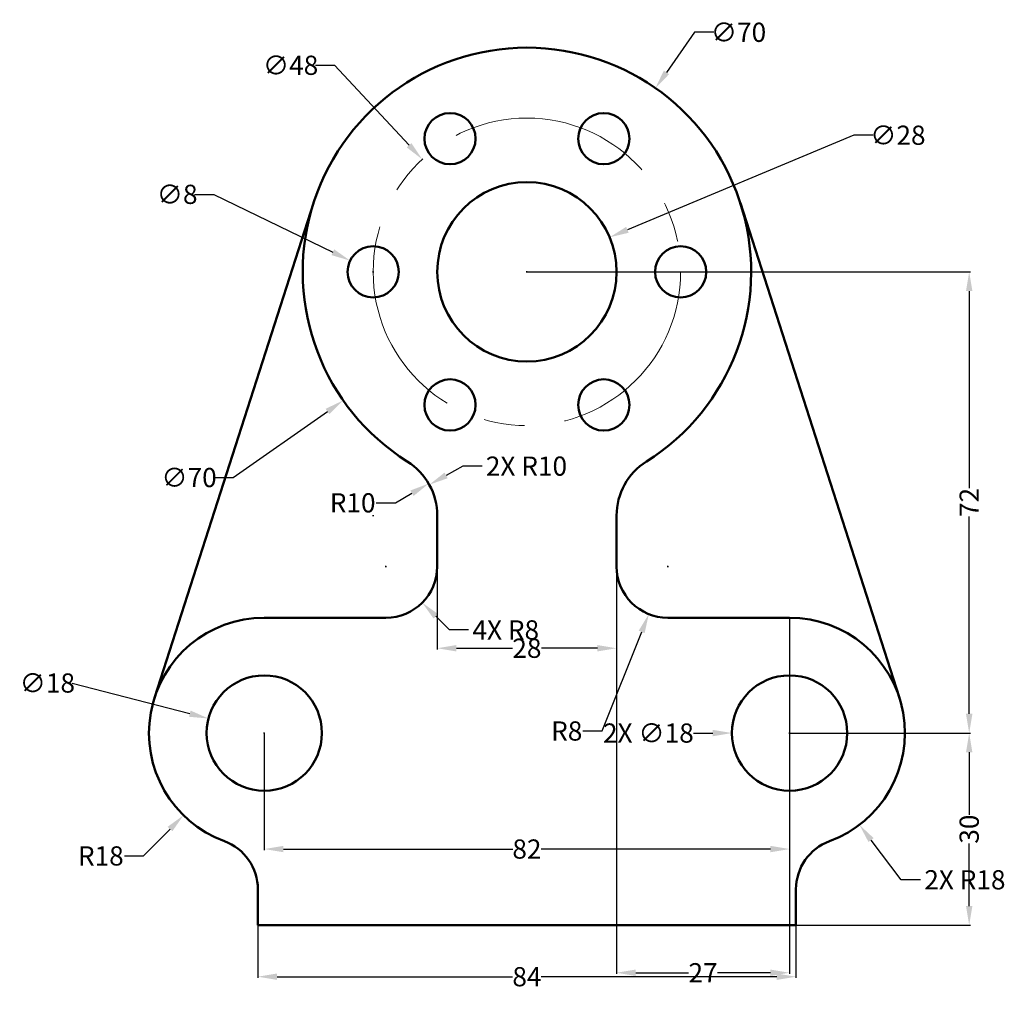
# Model space of a CAD drawing. Units: millimetres. Extents: x 5 to 159, y 16 to 167.
import ezdxf

# ---------------------------------------------------------------- set-up
doc = ezdxf.new("R2010")
doc.units = ezdxf.units.MM
doc.header["$MEASUREMENT"] = 0
doc.linetypes.add('CENTER', pattern=[50.8, 31.75, -6.35, 6.35, -6.35])
for name, color, linetype, lineweight in [('M-CNTR', 4, 'CENTER', 18), ('M-DIMS', 3, 'Continuous', 25), ('M-OUTL', 7, 'Continuous', 50)]:
    doc.layers.add(name, color=color, linetype=linetype, lineweight=lineweight)
doc.styles.get("Standard").update_dxf_attribs({"font": 'arial.ttf'})
doc.dimstyles.get("Standard").update_dxf_attribs({"dimtxt": 3, "dimasz": 3, "dimexe": 0.18, "dimexo": 0.0625, "dimgap": 0.09, "dimtad": 0, "dimtih": 1, "dimtoh": 1, "dimdec": 1, "dimdsep": 46, "dimtxsty": 'Standard', "dimcen": 0.09, "dimadec": 0, "dimazin": 0, "dimtfac": 1, "dimtdec": 1, "dimtofl": 0, "dimtmove": 0, "dimatfit": 3, "dimfxl": 1, "dimtolj": 1, "dimtzin": 0, "dimarcsym": 0})

# ---------------------------------------------------------------- blocks, each defined once
blk = doc.blocks.new('*D1')
at = {"layer": 'Defpoints', "color": 0, "transparency": 16777216}
for p in [(42.56, 25.69), (126.56, 25.69), (126.56, 17.65)]:
    blk.add_point(p, dxfattribs=at)
at = {"layer": 'M-DIMS', "color": 0, "lineweight": -2, "transparency": 16777216}
for p, q in [((42.56, 25.63), (42.56, 17.47)), ((126.56, 25.63), (126.56, 17.47)), ((45.56, 17.65), (82.33, 17.65)), ((123.56, 17.65), (86.8, 17.65))]:
    blk.add_line(p, q, dxfattribs=at)
at = {"layer": 'M-DIMS', "color": 0, "transparency": 16777216}
for points in [[(45.56, 18.15), (45.56, 17.15), (42.56, 17.65)], [(123.56, 18.15), (123.56, 17.15), (126.56, 17.65)]]:
    blk.add_solid(points, dxfattribs=at)
at = {"layer": 'M-DIMS', "color": 0, "transparency": 16777216, "insert": (84.56, 17.65), "char_height": 3, "attachment_point": 5}
blk.add_mtext('\\A1;84', dxfattribs=at)
blk = doc.blocks.new('*D2')
at = {"layer": 'Defpoints', "color": 0, "transparency": 16777216}
for p in [(43.56, 55.69), (125.56, 55.69), (125.56, 37.58)]:
    blk.add_point(p, dxfattribs=at)
at = {"layer": 'M-DIMS', "color": 0, "lineweight": -2, "transparency": 16777216}
for p, q in [((43.56, 55.63), (43.56, 37.4)), ((125.56, 55.63), (125.56, 37.4)), ((46.56, 37.58), (82.34, 37.58)), ((122.56, 37.58), (86.79, 37.58))]:
    blk.add_line(p, q, dxfattribs=at)
at = {"layer": 'M-DIMS', "color": 0, "transparency": 16777216}
for points in [[(46.56, 38.08), (46.56, 37.08), (43.56, 37.58)], [(122.56, 38.08), (122.56, 37.08), (125.56, 37.58)]]:
    blk.add_solid(points, dxfattribs=at)
at = {"layer": 'M-DIMS', "color": 0, "transparency": 16777216, "insert": (84.56, 37.58), "char_height": 3, "attachment_point": 5}
blk.add_mtext('\\A1;82', dxfattribs=at)
blk = doc.blocks.new('*D3')
at = {"layer": 'Defpoints', "color": 0, "transparency": 16777216}
for p in [(43.56, 55.69), (30.95, 42.85)]:
    blk.add_point(p, dxfattribs=at)
at = {"layer": 'M-DIMS', "color": 0, "lineweight": -2, "transparency": 16777216}
for p, q in [((43.47, 55.69), (43.65, 55.69)), ((43.56, 55.6), (43.56, 55.78)), ((24.73, 36.51), (28.85, 40.71)), ((21.73, 36.51), (24.73, 36.51))]:
    blk.add_line(p, q, dxfattribs=at)
at = {"layer": 'M-DIMS', "color": 0, "transparency": 16777216}
blk.add_solid([(28.49, 41.06), (29.21, 40.36), (30.95, 42.85)], dxfattribs=at)
at = {"layer": 'M-DIMS', "color": 0, "transparency": 16777216, "insert": (18.05, 36.51), "char_height": 3, "attachment_point": 5}
blk.add_mtext('\\A1;R18', dxfattribs=at)
blk = doc.blocks.new('*D4')
at = {"layer": 'Defpoints', "color": 0, "transparency": 16777216}
for p in [(34.85, 57.96), (52.27, 53.43)]:
    blk.add_point(p, dxfattribs=at)
at = {"layer": 'M-DIMS', "color": 0, "lineweight": -2, "transparency": 16777216}
for p, q in [((13.58, 63.5), (31.95, 58.72)), ((43.47, 55.69), (43.65, 55.69)), ((43.56, 55.6), (43.56, 55.78))]:
    blk.add_line(p, q, dxfattribs=at)
at = {"layer": 'M-DIMS', "color": 0, "transparency": 16777216}
blk.add_solid([(32.07, 59.2), (31.82, 58.23), (34.85, 57.96)], dxfattribs=at)
at = {"layer": 'M-DIMS', "color": 0, "transparency": 16777216, "insert": (9.7, 63.5), "char_height": 3, "attachment_point": 5}
blk.add_mtext('\\A1;∅18', dxfattribs=at)
blk = doc.blocks.new('*D5')
at = {"layer": 'Defpoints', "color": 0, "transparency": 16777216}
for p in [(125.56, 55.69), (153.6, 55.69), (126.56, 25.69)]:
    blk.add_point(p, dxfattribs=at)
at = {"layer": 'M-DIMS', "color": 0, "lineweight": -2, "transparency": 16777216}
for p, q in [((125.62, 55.69), (153.78, 55.69)), ((153.6, 52.69), (153.6, 42.93)), ((153.6, 28.69), (153.6, 38.46)), ((126.62, 25.69), (153.78, 25.69))]:
    blk.add_line(p, q, dxfattribs=at)
at = {"layer": 'M-DIMS', "color": 0, "transparency": 16777216}
for points in [[(153.1, 52.69), (154.1, 52.69), (153.6, 55.69)], [(153.1, 28.69), (154.1, 28.69), (153.6, 25.69)]]:
    blk.add_solid(points, dxfattribs=at)
at = {"layer": 'M-DIMS', "color": 0, "transparency": 16777216, "insert": (153.6, 40.69), "char_height": 3, "attachment_point": 5, "rotation": 90}
blk.add_mtext('\\A1;30', dxfattribs=at)
blk = doc.blocks.new('*D6')
at = {"layer": 'Defpoints', "color": 0, "transparency": 16777216}
for p in [(84.56, 127.69), (153.6, 127.69), (125.56, 55.69)]:
    blk.add_point(p, dxfattribs=at)
at = {"layer": 'M-DIMS', "color": 0, "lineweight": -2, "transparency": 16777216}
for p, q in [((84.62, 127.69), (153.78, 127.69)), ((153.6, 124.69), (153.6, 93.91)), ((153.6, 58.69), (153.6, 89.48)), ((125.62, 55.69), (153.78, 55.69))]:
    blk.add_line(p, q, dxfattribs=at)
at = {"layer": 'M-DIMS', "color": 0, "transparency": 16777216}
for points in [[(153.1, 124.69), (154.1, 124.69), (153.6, 127.69)], [(153.1, 58.69), (154.1, 58.69), (153.6, 55.69)]]:
    blk.add_solid(points, dxfattribs=at)
at = {"layer": 'M-DIMS', "color": 0, "transparency": 16777216, "insert": (153.6, 91.69), "char_height": 3, "attachment_point": 5, "rotation": 90}
blk.add_mtext('\\A1;72', dxfattribs=at)
blk = doc.blocks.new('*D7')
at = {"layer": 'Defpoints', "color": 0, "transparency": 16777216}
for p in [(70.56, 85.66), (98.56, 85.66), (98.56, 68.93)]:
    blk.add_point(p, dxfattribs=at)
at = {"layer": 'M-DIMS', "color": 0, "lineweight": -2, "transparency": 16777216}
for p, q in [((70.56, 85.6), (70.56, 68.75)), ((98.56, 85.6), (98.56, 68.75)), ((73.56, 68.93), (82.29, 68.93)), ((95.56, 68.93), (86.83, 68.93))]:
    blk.add_line(p, q, dxfattribs=at)
at = {"layer": 'M-DIMS', "color": 0, "transparency": 16777216}
for points in [[(73.56, 69.43), (73.56, 68.43), (70.56, 68.93)], [(95.56, 69.43), (95.56, 68.43), (98.56, 68.93)]]:
    blk.add_solid(points, dxfattribs=at)
at = {"layer": 'M-DIMS', "color": 0, "transparency": 16777216, "insert": (84.56, 68.93), "char_height": 3, "attachment_point": 5}
blk.add_mtext('\\A1;28', dxfattribs=at)
blk = doc.blocks.new('*D8')
at = {"layer": 'Defpoints', "color": 0, "transparency": 16777216}
for p in [(106.56, 81.69), (103.59, 74.27)]:
    blk.add_point(p, dxfattribs=at)
at = {"layer": 'M-DIMS', "color": 0, "lineweight": -2, "transparency": 16777216}
for p, q in [((106.47, 81.69), (106.65, 81.69)), ((106.56, 81.6), (106.56, 81.78)), ((96.29, 56.01), (102.48, 71.48)), ((93.29, 56.01), (96.29, 56.01))]:
    blk.add_line(p, q, dxfattribs=at)
at = {"layer": 'M-DIMS', "color": 0, "transparency": 16777216}
blk.add_solid([(102.01, 71.67), (102.94, 71.29), (103.59, 74.27)], dxfattribs=at)
at = {"layer": 'M-DIMS', "color": 0, "transparency": 16777216, "insert": (90.78, 56.01), "char_height": 3, "attachment_point": 5}
blk.add_mtext('\\A1;R8', dxfattribs=at)
blk = doc.blocks.new('*D9')
at = {"layer": 'Defpoints', "color": 0, "transparency": 16777216}
for p in [(69.22, 94.63), (60.56, 89.63)]:
    blk.add_point(p, dxfattribs=at)
at = {"layer": 'M-DIMS', "color": 0, "lineweight": -2, "transparency": 16777216}
for p, q in [((64.03, 91.63), (66.62, 93.13)), ((61.03, 91.63), (64.03, 91.63))]:
    blk.add_line(p, q, dxfattribs=at)
at = {"layer": 'M-DIMS', "color": 0, "transparency": 16777216}
blk.add_solid([(66.37, 93.56), (66.87, 92.7), (69.22, 94.63)], dxfattribs=at)
at = {"layer": 'M-DIMS', "color": 0, "transparency": 16777216, "insert": (57.36, 91.63), "char_height": 3, "attachment_point": 5}
blk.add_mtext('\\A1;R10', dxfattribs=at)
blk = doc.blocks.new('*D10')
at = {"layer": 'Defpoints', "color": 0, "transparency": 16777216}
for p in [(56.96, 129.44), (64.16, 125.95)]:
    blk.add_point(p, dxfattribs=at)
at = {"layer": 'M-DIMS', "color": 0, "lineweight": -2, "transparency": 16777216}
for p, q in [((32.67, 139.79), (35.67, 139.79)), ((35.67, 139.79), (54.27, 130.75)), ((60.47, 127.69), (60.65, 127.69)), ((60.56, 127.6), (60.56, 127.78))]:
    blk.add_line(p, q, dxfattribs=at)
at = {"layer": 'M-DIMS', "color": 0, "transparency": 16777216}
blk.add_solid([(54.48, 131.2), (54.05, 130.3), (56.96, 129.44)], dxfattribs=at)
at = {"layer": 'M-DIMS', "color": 0, "transparency": 16777216, "insert": (29.96, 139.79), "char_height": 3, "attachment_point": 5}
blk.add_mtext('\\A1;∅8', dxfattribs=at)
blk = doc.blocks.new('*D11')
at = {"layer": 'Defpoints', "color": 0, "transparency": 16777216}
for p in [(104.62, 156.37), (64.5, 99.02)]:
    blk.add_point(p, dxfattribs=at)
at = {"layer": 'M-DIMS', "color": 0, "lineweight": -2, "transparency": 16777216}
for p, q in [((110.72, 165.09), (106.34, 158.83)), ((113.72, 165.09), (110.72, 165.09)), ((84.47, 127.69), (84.65, 127.69)), ((84.56, 127.6), (84.56, 127.78))]:
    blk.add_line(p, q, dxfattribs=at)
at = {"layer": 'M-DIMS', "color": 0, "transparency": 16777216}
blk.add_solid([(105.93, 159.12), (106.75, 158.54), (104.62, 156.37)], dxfattribs=at)
at = {"layer": 'M-DIMS', "color": 0, "transparency": 16777216, "insert": (117.59, 165.09), "char_height": 3, "attachment_point": 5}
blk.add_mtext('\\A1;∅70', dxfattribs=at)
blk = doc.blocks.new('*D12')
at = {"layer": 'Defpoints', "color": 0, "transparency": 16777216}
for p in [(68.21, 145.26), (100.91, 110.13)]:
    blk.add_point(p, dxfattribs=at)
at = {"layer": 'M-DIMS', "color": 0, "lineweight": -2, "transparency": 16777216}
for p, q in [((51.54, 159.94), (54.54, 159.94)), ((54.54, 159.94), (66.16, 147.46)), ((84.47, 127.69), (84.65, 127.69)), ((84.56, 127.6), (84.56, 127.78))]:
    blk.add_line(p, q, dxfattribs=at)
at = {"layer": 'M-DIMS', "color": 0, "transparency": 16777216}
blk.add_solid([(66.53, 147.8), (65.8, 147.12), (68.21, 145.26)], dxfattribs=at)
at = {"layer": 'M-DIMS', "color": 0, "transparency": 16777216, "insert": (47.67, 159.94), "char_height": 3, "attachment_point": 5}
blk.add_mtext('\\A1;∅48', dxfattribs=at)
blk = doc.blocks.new('*D13')
at = {"layer": 'Defpoints', "color": 0, "transparency": 16777216}
for p in [(97.48, 133.09), (71.64, 122.3)]:
    blk.add_point(p, dxfattribs=at)
at = {"layer": 'M-DIMS', "color": 0, "lineweight": -2, "transparency": 16777216}
for p, q in [((135.59, 149.02), (100.25, 134.25)), ((138.59, 149.02), (135.59, 149.02)), ((84.47, 127.69), (84.65, 127.69)), ((84.56, 127.6), (84.56, 127.78))]:
    blk.add_line(p, q, dxfattribs=at)
at = {"layer": 'M-DIMS', "color": 0, "transparency": 16777216}
blk.add_solid([(100.05, 134.71), (100.44, 133.79), (97.48, 133.09)], dxfattribs=at)
at = {"layer": 'M-DIMS', "color": 0, "transparency": 16777216, "insert": (142.47, 149.02), "char_height": 3, "attachment_point": 5}
blk.add_mtext('\\A1;∅28', dxfattribs=at)
blk = doc.blocks.new('FLANGE-HOLE-D8')
blk.add_circle((4, 4), 4)
blk = doc.blocks.new('MOUNT-HOLE-D18')
blk.add_circle((9, 9), 9)
blk = doc.blocks.new('*D16')
at = {"layer": 'Defpoints', "color": 0, "transparency": 16777216}
for p in [(98.56, 81.69), (125.56, 73.69), (98.56, 18.27)]:
    blk.add_point(p, dxfattribs=at)
at = {"layer": 'M-DIMS', "color": 0, "lineweight": -2, "transparency": 16777216}
for p, q in [((98.56, 81.63), (98.56, 18.09)), ((125.56, 73.63), (125.56, 18.09)), ((101.56, 18.27), (109.8, 18.27)), ((122.56, 18.27), (114.33, 18.27))]:
    blk.add_line(p, q, dxfattribs=at)
at = {"layer": 'M-DIMS', "color": 0, "transparency": 16777216}
for points in [[(101.56, 18.77), (101.56, 17.77), (98.56, 18.27)], [(122.56, 18.77), (122.56, 17.77), (125.56, 18.27)]]:
    blk.add_solid(points, dxfattribs=at)
at = {"layer": 'M-DIMS', "color": 0, "transparency": 16777216, "insert": (112.06, 18.27), "char_height": 3, "attachment_point": 5}
blk.add_mtext('\\A1;27', dxfattribs=at)
blk = doc.blocks.new('*D17')
at = {"layer": 'Defpoints', "color": 0, "transparency": 16777216}
for p in [(113.23, 147.77), (55.89, 107.62)]:
    blk.add_point(p, dxfattribs=at)
at = {"layer": 'M-DIMS', "color": 0, "lineweight": -2, "transparency": 16777216}
for p, q in [((84.47, 127.69), (84.65, 127.69)), ((84.56, 127.6), (84.56, 127.78)), ((38.69, 95.58), (53.43, 105.9)), ((35.69, 95.58), (38.69, 95.58))]:
    blk.add_line(p, q, dxfattribs=at)
at = {"layer": 'M-DIMS', "color": 0, "transparency": 16777216}
blk.add_solid([(53.14, 106.31), (53.72, 105.49), (55.89, 107.62)], dxfattribs=at)
at = {"layer": 'M-DIMS', "color": 0, "transparency": 16777216, "insert": (31.82, 95.58), "char_height": 3, "attachment_point": 5}
blk.add_mtext('\\A1;∅70', dxfattribs=at)
blk = doc.blocks.new('*D18')
at = {"layer": 'Defpoints', "color": 0, "transparency": 16777216}
for p in [(69.32, 94.46), (60.56, 89.63)]:
    blk.add_point(p, dxfattribs=at)
at = {"layer": 'M-DIMS', "color": 0, "lineweight": -2, "transparency": 16777216}
for p, q in [((74.57, 97.36), (71.94, 95.91)), ((77.57, 97.36), (74.57, 97.36)), ((60.47, 89.63), (60.65, 89.63)), ((60.56, 89.54), (60.56, 89.72))]:
    blk.add_line(p, q, dxfattribs=at)
at = {"layer": 'M-DIMS', "color": 0, "transparency": 16777216}
blk.add_solid([(71.7, 96.35), (72.19, 95.47), (69.32, 94.46)], dxfattribs=at)
at = {"layer": 'M-DIMS', "color": 0, "transparency": 16777216, "insert": (84.49, 97.36), "char_height": 3, "attachment_point": 5}
blk.add_mtext('\\A1;2X R10', dxfattribs=at)
blk = doc.blocks.new('*D19')
at = {"layer": 'Defpoints', "color": 0, "transparency": 16777216}
for p in [(62.56, 81.69), (68.22, 76.04)]:
    blk.add_point(p, dxfattribs=at)
at = {"layer": 'M-DIMS', "color": 0, "lineweight": -2, "transparency": 16777216}
for p, q in [((62.47, 81.69), (62.65, 81.69)), ((62.56, 81.6), (62.56, 81.78)), ((72.46, 71.79), (70.34, 73.92)), ((75.46, 71.79), (72.46, 71.79))]:
    blk.add_line(p, q, dxfattribs=at)
at = {"layer": 'M-DIMS', "color": 0, "transparency": 16777216}
blk.add_solid([(70.69, 74.27), (69.99, 73.56), (68.22, 76.04)], dxfattribs=at)
at = {"layer": 'M-DIMS', "color": 0, "transparency": 16777216, "insert": (81.26, 71.79), "char_height": 3, "attachment_point": 5}
blk.add_mtext('\\A1;4X R8', dxfattribs=at)
blk = doc.blocks.new('*D20')
at = {"layer": 'Defpoints', "color": 0, "transparency": 16777216}
for p in [(125.56, 55.69), (136.46, 41.37)]:
    blk.add_point(p, dxfattribs=at)
at = {"layer": 'M-DIMS', "color": 0, "lineweight": -2, "transparency": 16777216}
for p, q in [((125.47, 55.69), (125.65, 55.69)), ((125.56, 55.6), (125.56, 55.78)), ((143, 32.78), (138.28, 38.98)), ((146, 32.78), (143, 32.78))]:
    blk.add_line(p, q, dxfattribs=at)
at = {"layer": 'M-DIMS', "color": 0, "transparency": 16777216}
blk.add_solid([(138.68, 39.29), (137.88, 38.68), (136.46, 41.37)], dxfattribs=at)
at = {"layer": 'M-DIMS', "color": 0, "transparency": 16777216, "insert": (152.93, 32.78), "char_height": 3, "attachment_point": 5}
blk.add_mtext('\\A1;2X R18', dxfattribs=at)
blk = doc.blocks.new('*D21')
at = {"layer": 'Defpoints', "color": 0, "transparency": 16777216}
for p in [(116.56, 55.69), (134.56, 55.69)]:
    blk.add_point(p, dxfattribs=at)
at = {"layer": 'M-DIMS', "color": 0, "lineweight": -2, "transparency": 16777216}
for p, q in [((110.56, 55.69), (113.56, 55.69)), ((125.47, 55.69), (125.65, 55.69)), ((125.56, 55.6), (125.56, 55.78))]:
    blk.add_line(p, q, dxfattribs=at)
at = {"layer": 'M-DIMS', "color": 0, "transparency": 16777216}
blk.add_solid([(113.56, 56.19), (113.56, 55.19), (116.56, 55.69)], dxfattribs=at)
at = {"layer": 'M-DIMS', "color": 0, "transparency": 16777216, "insert": (103.52, 55.69), "char_height": 3, "attachment_point": 5}
blk.add_mtext('\\A1;2X ∅18', dxfattribs=at)

msp = doc.modelspace()

# ---------------------------------------------------------------- linework, layer by layer
at = {"layer": 'M-CNTR'}
msp.add_circle((84.56, 127.69), 24, dxfattribs=at)
at = {"layer": 'M-OUTL'}
for p, q in [((26.42, 61.2), (51.24, 138.4)), ((142.7, 61.2), (117.88, 138.4)), ((70.56, 89.63), (70.56, 81.69)), ((98.56, 89.63), (98.56, 81.69)), ((43.56, 73.69), (62.56, 73.69)), ((106.56, 73.69), (125.56, 73.69)), ((42.56, 25.69), (42.56, 31.3)), ((126.56, 25.69), (126.56, 31.3)), ((43.56, 25.69), (42.56, 25.69)), ((43.56, 25.69), (125.56, 25.69)), ((125.56, 25.69), (126.56, 25.69))]:
    msp.add_line(p, q, dxfattribs=at)
msp.add_circle((84.56, 127.69), 14, dxfattribs=at)
for centre, radius, start, end in [((84.56, 127.69), 35, 302.231, 237.769), ((60.56, 89.63), 10, 0, 57.769), ((108.56, 89.63), 10, 122.231, 180), ((62.56, 81.69), 8, 270, 0), ((106.56, 81.69), 8, 180, 270), ((43.56, 55.69), 18, 90, 249.7478), ((125.56, 55.69), 18, 290.2522, 90), ((34.56, 31.3), 8, 0, 69.7478), ((134.56, 31.3), 8, 110.2522, 180)]:
    msp.add_arc(centre, radius, start, end, dxfattribs=at)

# ---------------------------------------------------------------- block references
for name, p in [('FLANGE-HOLE-D8', (68.56, 144.48)), ('FLANGE-HOLE-D8', (92.56, 144.48)), ('FLANGE-HOLE-D8', (56.56, 123.69)), ('FLANGE-HOLE-D8', (104.56, 123.69)), ('FLANGE-HOLE-D8', (68.56, 102.91)), ('FLANGE-HOLE-D8', (92.56, 102.91)), ('MOUNT-HOLE-D18', (34.56, 46.69)), ('MOUNT-HOLE-D18', (116.56, 46.69))]:
    msp.add_blockref(name, p, dxfattribs=at)

# ---------------------------------------------------------------- dimensions: what is measured, and where the dimension line sits
at = {"layer": 'M-DIMS', "transparency": 33554610}
for p1, p2, picture, middle in [((64.5, 99.02), (104.62, 156.37), '*D11', (117.59, 165.09)), ((100.91, 110.13), (68.21, 145.26), '*D12', (47.67, 159.94)), ((71.64, 122.3), (97.48, 133.09), '*D13', (142.47, 149.02)), ((64.16, 125.95), (56.96, 129.44), '*D10', (29.96, 139.79)), ((52.27, 53.43), (34.85, 57.96), '*D4', (13.58, 63.5))]:
    dim = msp.add_diameter_dim_2p(p1=p1, p2=p2, dimstyle='Standard', override={"dimclrd": 0, "dimclre": 0, "dimclrt": 0}, dxfattribs=at)
    dim.commit()
    dim.dimension.update_dxf_attribs({"geometry": picture, "text_midpoint": middle, "dimtype": 163})
at = {"layer": 'M-DIMS'}
dim = msp.add_diameter_dim_2p(p1=(113.23, 147.77), p2=(55.89, 107.62), dimstyle='Standard', override={"dimdec": 0, "dimlfac": 1, "dimrnd": 0, "dimzin": 0, "dimdsep": 46, "dimlunit": 2}, dxfattribs=at)
dim.commit()
dim.dimension.update_dxf_attribs({"geometry": '*D17', "text_midpoint": (31.82, 95.58), "dimtype": 163})
at = {"layer": 'M-DIMS', "transparency": 33554610}
for base, p1, p2, picture, middle in [((153.6, 127.69), (125.56, 55.69), (84.56, 127.69), '*D6', (153.6, 91.69)), ((153.6, 55.69), (126.56, 25.69), (125.56, 55.69), '*D5', (153.6, 40.69))]:
    dim = msp.add_linear_dim(base=base, p1=p1, p2=p2, angle=90, dimstyle='Standard', override={"dimclrd": 0, "dimclre": 0, "dimclrt": 0}, dxfattribs=at)
    dim.commit()
    dim.dimension.update_dxf_attribs({"geometry": picture, "text_midpoint": middle, "text_rotation": 90})
at = {"layer": 'M-DIMS'}
for center, mpoint, picture, middle in [((60.56, 89.63), (69.32, 94.46), '*D18', (84.49, 97.36)), ((125.56, 55.69), (136.46, 41.37), '*D20', (152.93, 32.78))]:
    dim = msp.add_radius_dim(center=center, mpoint=mpoint, text='2X <>', dimstyle='Standard', override={"dimdec": 0, "dimlfac": 1, "dimrnd": 0, "dimzin": 0, "dimdsep": 46, "dimlunit": 2}, dxfattribs=at)
    dim.commit()
    dim.dimension.update_dxf_attribs({"geometry": picture, "text_midpoint": middle, "dimtype": 164})
at = {"layer": 'M-DIMS', "transparency": 33554610}
for center, mpoint, picture, middle in [((60.56, 89.63), (69.22, 94.63), '*D9', (57.36, 91.63)), ((106.56, 81.69), (103.59, 74.27), '*D8', (90.78, 56.01)), ((43.56, 55.69), (30.95, 42.85), '*D3', (18.05, 36.51))]:
    dim = msp.add_radius_dim(center=center, mpoint=mpoint, dimstyle='Standard', override={"dimclrd": 0, "dimclre": 0, "dimclrt": 0}, dxfattribs=at)
    dim.commit()
    dim.dimension.update_dxf_attribs({"geometry": picture, "text_midpoint": middle, "dimtype": 164})
for base, p1, p2, picture, middle in [((98.56, 68.93), (70.56, 85.66), (98.56, 85.66), '*D7', (84.56, 68.93)), ((125.56, 37.58), (43.56, 55.69), (125.56, 55.69), '*D2', (84.56, 37.58)), ((126.56, 17.65), (42.56, 25.69), (126.56, 25.69), '*D1', (84.56, 17.65))]:
    dim = msp.add_linear_dim(base=base, p1=p1, p2=p2, dimstyle='Standard', override={"dimclrd": 0, "dimclre": 0, "dimclrt": 0}, dxfattribs=at)
    dim.commit()
    dim.dimension.update_dxf_attribs({"geometry": picture, "text_midpoint": middle})
at = {"layer": 'M-DIMS'}
dim = msp.add_radius_dim(center=(62.56, 81.69), mpoint=(68.22, 76.04), text='4X <>', dimstyle='Standard', override={"dimdec": 0, "dimlfac": 1, "dimrnd": 0, "dimzin": 0, "dimdsep": 46, "dimlunit": 2}, dxfattribs=at)
dim.commit()
dim.dimension.update_dxf_attribs({"geometry": '*D19', "text_midpoint": (81.26, 71.79)})
dim = msp.add_linear_dim(base=(98.56, 18.27), p1=(125.56, 73.69), p2=(98.56, 81.69), dimstyle='Standard', override={"dimdec": 0, "dimlfac": 1, "dimrnd": 0, "dimzin": 0, "dimdsep": 46, "dimlunit": 2}, dxfattribs=at)
dim.commit()
dim.dimension.update_dxf_attribs({"geometry": '*D16', "text_midpoint": (112.06, 18.27)})
dim = msp.add_diameter_dim_2p(p1=(134.56, 55.69), p2=(116.56, 55.69), text='2X <>', dimstyle='Standard', override={"dimdec": 0, "dimlfac": 1, "dimrnd": 0, "dimzin": 0, "dimdsep": 46, "dimlunit": 2}, dxfattribs=at)
dim.commit()
dim.dimension.update_dxf_attribs({"geometry": '*D21', "text_midpoint": (110.56, 55.69), "dimtype": 163})

doc.saveas('drawing.dxf')
